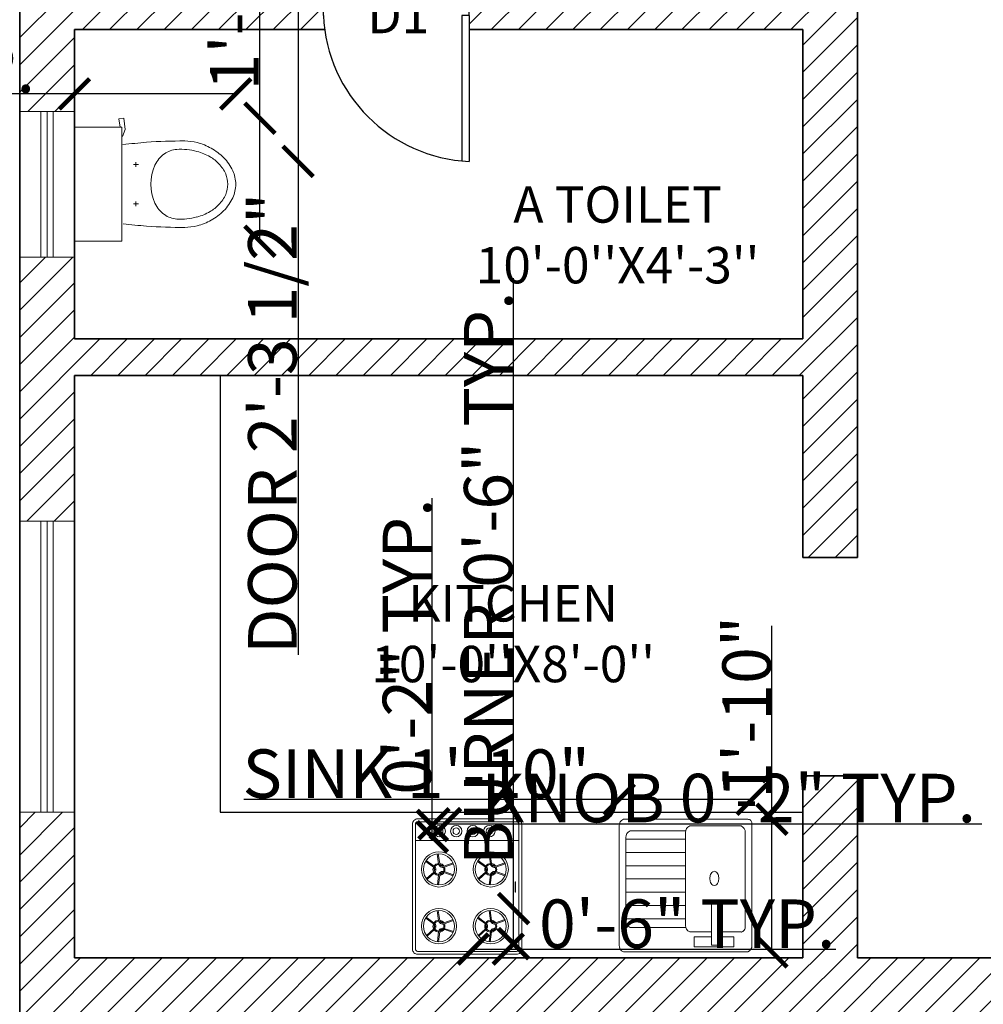
# Model space of a CAD drawing. Units: inches. Extents: x 2094 to 2639, y 1426 to 1997.
# Tile 3 of 8: x 2180 to 2339, y 1567 to 1730. Entities that reach past the tile are written whole.
import ezdxf

# ---------------------------------------------------------------- set-up
doc = ezdxf.new("R2010")
doc.units = ezdxf.units.IN
for name, color, linetype, lineweight in [('A-ANNO-DIMS', 2, 'Continuous', 18), ('A-ANNO-TEXT', 7, 'Continuous', 18), ('A-AREA-IDEN', 7, 'Continuous', 25), ('A-EQPM', 9, 'Continuous', 13), ('A-FLOR-FIXT', 9, 'Continuous', 18), ('A-WALL-PATT', 8, 'Continuous', 13), ('Doors', 34, 'Continuous', 25), ('Kitchen', 70, 'Continuous', 25), ('Walls', 7, 'Continuous', 35), ('Windows', 150, 'Continuous', 18)]:
    doc.layers.add(name, color=color, linetype=linetype, lineweight=lineweight)
doc.styles.get("Standard").update_dxf_attribs({"font": 'arial.ttf'})
doc.dimstyles.get("Standard").update_dxf_attribs({"dimtxt": 8, "dimasz": 5, "dimexe": 0.18, "dimexo": 0.0625, "dimgap": 0.09, "dimtad": 1, "dimdec": 1, "dimzin": 0, "dimdsep": 46, "dimlunit": 4, "dimtxsty": 'Standard', "dimblk": 'ARCHTICK', "dimcen": 0.09, "dimse1": 1, "dimse2": 1, "dimadec": 0, "dimazin": 0, "dimtfac": 1, "dimtdec": 1, "dimtofl": 0, "dimtmove": 0, "dimatfit": 3, "dimfxl": 1, "dimtolj": 1, "dimtzin": 0, "dimarcsym": 0})

# ---------------------------------------------------------------- blocks, each defined once
blk = doc.blocks.new('toilet-1')
at = {"color": 0, "linetype": 'ByBlock'}
for p, q in [((-0.23, -0.02), (-0.23, -0.2116)), ((0.23, -0.02), (-0.23, -0.02)), ((0.23, -0.02), (0.23, -0.2116)), ((-0.23, -0.2116), (0.23, -0.2116)), ((0.1917, -0.2144), (0.2206, -0.225)), ((0.2206, -0.225), (0.266, -0.2187)), ((0.2633, -0.1997), (0.23, -0.2044)), ((0.266, -0.2187), (0.2633, -0.1997)), ((-0.0889, -0.2683), (-0.0697, -0.2683)), ((-0.0793, -0.2587), (-0.0793, -0.2778)), ((0.0889, -0.2683), (0.0698, -0.2683)), ((0.0794, -0.2587), (0.0794, -0.2778)), ((0, -0.6382), (0, -0.6382))]:
    blk.add_line(p, q, dxfattribs=at)
for centre, radius, start, end in [((3.5272, -0.6239), 3.7093, 173.6925, 175.1593), ((-3.527, -0.624), 3.7093, 4.8413, 6.3171), ((1.7368, -0.4519), 1.9109, 175.7698, 180.3758), ((-1.7366, -0.4519), 1.9109, 359.6242, 4.2302), ((-0.0312, -0.4465), 0.1114, 113.8997, 145.1485), ((0, -0.5169), 0.1884, 66.0939, 113.9061), ((0.0312, -0.4465), 0.1114, 34.8515, 66.1003), ((-0.0408, -0.4398), 0.0996, 145.1497, 175.881), ((0.0409, -0.4398), 0.0996, 4.119, 34.8503), ((0.0981, -0.4497), 0.2389, 175.8862, 195.5931), ((-0.098, -0.4497), 0.2389, 344.4069, 4.1138), ((0.0353, -0.463), 0.2093, 180.3747, 194.3375), ((-0.0351, -0.463), 0.2093, 345.6614, 359.6243), ((0.055, -0.458), 0.2297, 194.3353, 209.622), ((0.0961, -0.4503), 0.2369, 195.5969, 209.3771), ((-0.096, -0.4503), 0.2369, 330.6229, 344.4031), ((-0.0548, -0.458), 0.2297, 330.3788, 345.6655), ((0.0647, -0.4524), 0.2409, 209.6273, 224.5489), ((0.0232, -0.4913), 0.1532, 209.3871, 226.5438), ((-0.0231, -0.4913), 0.1532, 313.4562, 330.6129), ((-0.0645, -0.4524), 0.2409, 315.4504, 330.372), ((0.0178, -0.4986), 0.1751, 224.552, 245.714), ((0.0152, -0.4997), 0.1416, 226.5501, 246.5527), ((0, -0.5347), 0.1034, 246.5493, 270.0042), ((0, -0.5347), 0.1034, 269.9958, 293.4507), ((-0.0151, -0.4997), 0.1416, 293.4473, 313.4499), ((-0.0176, -0.4986), 0.1751, 294.2865, 315.4485), ((0.0004, -0.538), 0.132, 245.5845, 269.8782), ((-0.0002, -0.538), 0.132, 270.1216, 294.4153)]:
    blk.add_arc(centre, radius, start, end, dxfattribs=at)
blk = doc.blocks.new('S_SINK12')
for p, q in [((0.25, 0.45), (0.25, 0.0004)), ((0.35, 0.45), (0.35, 0.0004)), ((0.45, 0.45), (0.45, 0.0004)), ((0.55, 0.45), (0.55, 0.0004)), ((0.65, 0.45), (0.65, 0.0004)), ((0.75, 0.45), (0.75, 0.0004)), ((0.85, 0.45), (0.85, 0.0004))]:
    blk.add_line(p, q)
for points in [[(0, -0.4688), (0, 0.4688, -0.310961), (0.05, 0.4998), (0.95, 0.4998, -0.310466), (1, 0.4686), (1, -0.4688, -0.414214), (0.9687, -0.5), (0.05, -0.5002, -0.309971)], [(0.0516, -0.1954), (0.0516, -0.242), (0.3617, -0.242, 1), (0.3617, -0.1954)], [(0.4997, -0.2171), (0.5033, -0.2291, 0.107136), (0.5156, -0.241, 0.076468), (0.5341, -0.249), (0.5538, -0.2509), (0.5755, -0.2481, 0.076468), (0.5921, -0.241, 0.107136), (0.6044, -0.2291), (0.608, -0.2171), (0.6044, -0.2051, 0.107136), (0.5921, -0.1931, 0.076468), (0.5755, -0.186), (0.5538, -0.1832), (0.5322, -0.186, 0.076468), (0.5156, -0.1931, 0.107136), (0.5033, -0.2051)]]:
    blk.add_lwpolyline(points, format="xyb", close=True)
for points in [[(0.1851, -0.001), (0.1851, 0.4188, -0.310466), (0.2351, 0.45), (0.8621, 0.45, -0.310466), (0.9121, 0.4188), (0.9121, -0.0005, -0.310466)], [(0.15, -0.1954), (0.15, -0.0308, -0.310466), (0.2, 0.0004), (0.9, 0.0004, -0.310466), (0.95, -0.0308), (0.95, -0.4189, -0.310466), (0.9, -0.4502), (0.2, -0.4502), (0.1799, -0.4479, -0.071009), (0.1646, -0.4419, -0.106323), (0.1531, -0.4318), (0.1499, -0.422), (0.1508, -0.4192)]]:
    blk.add_lwpolyline(points, format="xyb")
for points in [[(0.1136, -0.242), (0.1136, -0.3644), (0.0386, -0.3644), (0.0386, -0.0644), (0.1136, -0.0644), (0.1136, -0.1954)], [(0.15, -0.4189), (0.15, -0.242)]]:
    blk.add_lwpolyline(points)
blk = doc.blocks.new('AP0B05')
for p, q in [((35, 100), (35, 880)), ((75, 100), (75, 878.9)), ((35, 100), (35, -20)), ((815, 100), (815, -20))]:
    blk.add_line(p, q)
blk.add_lwpolyline([(35, 100), (75, 100)])
blk.add_arc((-2.4, 62.6), 818.3, 2.6212, 87.3788)
blk = doc.blocks.new('_ArchTick')
at = {"color": 0, "linetype": 'ByBlock', "const_width": 0.15}
blk.add_lwpolyline([(-0.5, -0.5), (0.5, 0.5)], dxfattribs=at)
blk = doc.blocks.new('*D14')
at = {"layer": 'A-ANNO-DIMS', "color": 0, "lineweight": -2, "transparency": 16777216}
blk.add_line((2154, 1928.9), (2154, 1459.9), dxfattribs=at)
at = {"layer": 'Defpoints', "color": 0, "transparency": 16777216}
for p in [(2180.06, 1928.9), (2154, 1459.9), (2180.06, 1459.9)]:
    blk.add_point(p, dxfattribs=at)
at = {"layer": 'A-ANNO-DIMS', "color": 0, "lineweight": -2, "transparency": 16777216, "xscale": 5, "yscale": 5, "zscale": 5}
for p, rotation in [((2154, 1928.9), 90), ((2154, 1459.9), 270)]:
    blk.add_blockref('_ArchTick', p, dxfattribs=dict(at, rotation=rotation))
at = {"layer": 'A-ANNO-DIMS', "color": 0, "transparency": 16777216, "insert": (2149.82, 1694.4), "char_height": 8, "attachment_point": 5, "rotation": 90}
blk.add_mtext('\\A1;39\'-1"', dxfattribs=at)
blk = doc.blocks.new('COOKTOP-BURNER')
for points in [[(-0.28, 2.54), (-0.05, 0.93, 0.472479), (0.86, 0.37), (2.39, 0.92)], [(-0.11, 2.56), (0.12, 0.95, 0.472071), (0.81, 0.53), (2.32, 1.08)], [(-2.06, -1.52), (-0.85, -0.44, 0.472071), (-0.89, 0.37), (-2.19, 1.33)], [(-1.95, -1.65), (-0.74, -0.56, 0.472479), (-0.79, 0.51), (-2.09, 1.47)], [(-0.26, -2.54), (-0.05, -0.93, -0.472479), (0.87, -0.36), (2.39, -0.9)], [(-0.09, -2.56), (0.12, -0.95, -0.472071), (0.81, -0.52), (2.33, -1.06)]]:
    blk.add_lwpolyline(points, format="xyb")
for radius in [2.9, 2.56]:
    blk.add_circle((0, 0), radius)
for radius, start, end in [(0.989, 156.9326, 207.478), (0.989, 93.6067, 146.9387), (0.818, 161.7394, 202.6344), (0.818, 92.012, 148.4601), (0.989, 33.0309, 83.5763), (0.818, 37.8377, 78.7328), (0.818, 335.9407, 24.5584), (0.989, 337.462, 23.0371), (0.989, 217.5084, 266.8924), (0.818, 215.9137, 268.4871), (0.989, 276.9228, 327.4682), (0.818, 281.7663, 322.6614)]:
    blk.add_arc((0, 0), radius, start, end)
blk = doc.blocks.new('COOKTOP-KNOB')
for radius in [0.938, 0.533]:
    blk.add_circle((0, 0), radius)
blk = doc.blocks.new('*D23')
at = {"layer": 'A-ANNO-DIMS', "color": 0, "lineweight": -2, "transparency": 16777216}
for p, q in [((2225.93, 1733.9), (2225.93, 1706.16)), ((2225.93, 1706.16), (2225.93, 1624.84))]:
    blk.add_line(p, q, dxfattribs=at)
at = {"layer": 'Defpoints', "color": 0, "transparency": 16777216}
for p in [(2230.09, 1733.9), (2225.93, 1706.16), (2230.09, 1706.16)]:
    blk.add_point(p, dxfattribs=at)
at = {"layer": 'A-ANNO-DIMS', "color": 0, "lineweight": -2, "transparency": 16777216, "xscale": 5, "yscale": 5, "zscale": 5}
for p, rotation in [((2225.93, 1733.9), 90), ((2225.93, 1706.16), 270)]:
    blk.add_blockref('_ArchTick', p, dxfattribs=dict(at, rotation=rotation))
at = {"layer": 'A-ANNO-DIMS', "color": 0, "transparency": 16777216, "insert": (2221.69, 1663), "char_height": 8, "attachment_point": 5, "rotation": 90}
blk.add_mtext('\\A1;DOOR 2\'-3 1/2"', dxfattribs=at)
blk = doc.blocks.new('*D39')
at = {"layer": 'A-ANNO-DIMS', "color": 0, "lineweight": -2, "transparency": 16777216}
for p, q in [((2189.06, 1717.27), (2094.42, 1717.27)), ((2215.64, 1717.27), (2189.06, 1717.27))]:
    blk.add_line(p, q, dxfattribs=at)
at = {"layer": 'Defpoints', "color": 0, "transparency": 16777216}
for p in [(2189.06, 1717.27), (2189.06, 1713.28), (2215.64, 1713.28)]:
    blk.add_point(p, dxfattribs=at)
at = {"layer": 'A-ANNO-DIMS', "color": 0, "lineweight": -2, "transparency": 16777216, "xscale": 5, "yscale": 5, "zscale": 5, "rotation": 180}
blk.add_blockref('_ArchTick', (2189.06, 1717.27), dxfattribs=at)
at = {"layer": 'A-ANNO-DIMS', "color": 0, "lineweight": -2, "transparency": 16777216, "xscale": 5, "yscale": 5, "zscale": 5}
blk.add_blockref('_ArchTick', (2215.64, 1717.27), dxfattribs=at)
at = {"layer": 'A-ANNO-DIMS', "color": 0, "transparency": 16777216, "insert": (2139.24, 1721.49), "char_height": 8, "attachment_point": 5}
blk.add_mtext('\\A1;WC 2\'-2 1/2" TYP.', dxfattribs=at)
blk = doc.blocks.new('*D40')
at = {"layer": 'A-ANNO-DIMS', "color": 0, "lineweight": -2, "transparency": 16777216}
for p, q in [((2219.63, 1713.28), (2219.63, 1785.11)), ((2219.63, 1692.99), (2219.63, 1713.28))]:
    blk.add_line(p, q, dxfattribs=at)
at = {"layer": 'Defpoints', "color": 0, "transparency": 16777216}
for p in [(2215.64, 1713.28), (2219.63, 1713.28), (2215.64, 1692.99)]:
    blk.add_point(p, dxfattribs=at)
at = {"layer": 'A-ANNO-DIMS', "color": 0, "lineweight": -2, "transparency": 16777216, "xscale": 5, "yscale": 5, "zscale": 5}
for p, rotation in [((2219.63, 1713.28), 90), ((2219.63, 1692.99), 270)]:
    blk.add_blockref('_ArchTick', p, dxfattribs=dict(at, rotation=rotation))
at = {"layer": 'A-ANNO-DIMS', "color": 0, "transparency": 16777216, "insert": (2215.41, 1751.7), "char_height": 8, "attachment_point": 5, "rotation": 90}
blk.add_mtext('\\A1;1\'-8 1/2" TYP.', dxfattribs=at)
blk = doc.blocks.new('*D41')
at = {"layer": 'A-ANNO-DIMS', "color": 0, "lineweight": -2, "transparency": 16777216}
for p, q in [((2261.42, 1583.02), (2261.42, 1686.91)), ((2261.42, 1577.23), (2261.42, 1583.02))]:
    blk.add_line(p, q, dxfattribs=at)
at = {"layer": 'Defpoints', "color": 0, "transparency": 16777216}
for p in [(2260.56, 1583.02), (2261.42, 1583.02), (2260.56, 1577.23)]:
    blk.add_point(p, dxfattribs=at)
at = {"layer": 'A-ANNO-DIMS', "color": 0, "lineweight": -2, "transparency": 16777216, "xscale": 5, "yscale": 5, "zscale": 5}
for p, rotation in [((2261.42, 1583.02), 90), ((2261.42, 1577.23), 270)]:
    blk.add_blockref('_ArchTick', p, dxfattribs=dict(at, rotation=rotation))
at = {"layer": 'A-ANNO-DIMS', "color": 0, "transparency": 16777216, "insert": (2257.25, 1637.47), "char_height": 8, "attachment_point": 5, "rotation": 90}
blk.add_mtext('\\A1;BURNER 0\'-6" TYP.', dxfattribs=at)
blk = doc.blocks.new('*D42')
at = {"layer": 'A-ANNO-DIMS', "color": 0, "lineweight": -2, "transparency": 16777216}
for p, q in [((2254.76, 1576.36), (2260.56, 1576.36)), ((2260.56, 1576.36), (2314.5, 1576.36))]:
    blk.add_line(p, q, dxfattribs=at)
at = {"layer": 'Defpoints', "color": 0, "transparency": 16777216}
for p in [(2254.76, 1577.23), (2260.56, 1577.23), (2260.56, 1576.36)]:
    blk.add_point(p, dxfattribs=at)
at = {"layer": 'A-ANNO-DIMS', "color": 0, "lineweight": -2, "transparency": 16777216, "xscale": 5, "yscale": 5, "zscale": 5, "rotation": 180}
blk.add_blockref('_ArchTick', (2254.76, 1576.36), dxfattribs=at)
at = {"layer": 'A-ANNO-DIMS', "color": 0, "lineweight": -2, "transparency": 16777216, "xscale": 5, "yscale": 5, "zscale": 5}
blk.add_blockref('_ArchTick', (2260.56, 1576.36), dxfattribs=at)
at = {"layer": 'A-ANNO-DIMS', "color": 0, "transparency": 16777216, "insert": (2290.03, 1580.53), "char_height": 8, "attachment_point": 5}
blk.add_mtext('\\A1;0\'-6" TYP.', dxfattribs=at)
blk = doc.blocks.new('*D43')
at = {"layer": 'A-ANNO-DIMS', "color": 0, "lineweight": -2, "transparency": 16777216}
for p, q in [((2248.31, 1597.01), (2250.19, 1597.01)), ((2250.19, 1597.01), (2338.56, 1597.01))]:
    blk.add_line(p, q, dxfattribs=at)
at = {"layer": 'Defpoints', "color": 0, "transparency": 16777216}
for p in [(2248.31, 1596.73), (2250.19, 1597.01), (2250.19, 1596.73)]:
    blk.add_point(p, dxfattribs=at)
at = {"layer": 'A-ANNO-DIMS', "color": 0, "lineweight": -2, "transparency": 16777216, "xscale": 5, "yscale": 5, "zscale": 5, "rotation": 180}
blk.add_blockref('_ArchTick', (2248.31, 1597.01), dxfattribs=at)
at = {"layer": 'A-ANNO-DIMS', "color": 0, "lineweight": -2, "transparency": 16777216, "xscale": 5, "yscale": 5, "zscale": 5}
blk.add_blockref('_ArchTick', (2250.19, 1597.01), dxfattribs=at)
at = {"layer": 'A-ANNO-DIMS', "color": 0, "transparency": 16777216, "insert": (2296.87, 1601.24), "char_height": 8, "attachment_point": 5}
blk.add_mtext('\\A1;KNOB 0\'-2" TYP.', dxfattribs=at)
blk = doc.blocks.new('*D44')
at = {"layer": 'A-ANNO-DIMS', "color": 0, "lineweight": -2, "transparency": 16777216}
for p, q in [((2248.03, 1596.73), (2248.03, 1650.68)), ((2248.03, 1594.86), (2248.03, 1596.73))]:
    blk.add_line(p, q, dxfattribs=at)
at = {"layer": 'Defpoints', "color": 0, "transparency": 16777216}
for p in [(2248.03, 1596.73), (2248.31, 1596.73), (2248.31, 1594.86)]:
    blk.add_point(p, dxfattribs=at)
at = {"layer": 'A-ANNO-DIMS', "color": 0, "lineweight": -2, "transparency": 16777216, "xscale": 5, "yscale": 5, "zscale": 5}
for p, rotation in [((2248.03, 1596.73), 90), ((2248.03, 1594.86), 270)]:
    blk.add_blockref('_ArchTick', p, dxfattribs=dict(at, rotation=rotation))
at = {"layer": 'A-ANNO-DIMS', "color": 0, "transparency": 16777216, "insert": (2243.86, 1626.2), "char_height": 8, "attachment_point": 5, "rotation": 90}
blk.add_mtext('\\A1;0\'-2" TYP.', dxfattribs=at)
blk = doc.blocks.new('*D45')
at = {"layer": 'A-ANNO-DIMS', "color": 0, "lineweight": -2, "transparency": 16777216}
for p, q in [((2278.81, 1601.03), (2217, 1601.03)), ((2300.71, 1601.03), (2278.81, 1601.03))]:
    blk.add_line(p, q, dxfattribs=at)
at = {"layer": 'Defpoints', "color": 0, "transparency": 16777216}
for p in [(2278.81, 1601.03), (2278.81, 1597.75), (2300.71, 1597.75)]:
    blk.add_point(p, dxfattribs=at)
at = {"layer": 'A-ANNO-DIMS', "color": 0, "lineweight": -2, "transparency": 16777216, "xscale": 5, "yscale": 5, "zscale": 5, "rotation": 180}
blk.add_blockref('_ArchTick', (2278.81, 1601.03), dxfattribs=at)
at = {"layer": 'A-ANNO-DIMS', "color": 0, "lineweight": -2, "transparency": 16777216, "xscale": 5, "yscale": 5, "zscale": 5}
blk.add_blockref('_ArchTick', (2300.71, 1601.03), dxfattribs=at)
at = {"layer": 'A-ANNO-DIMS', "color": 0, "transparency": 16777216, "insert": (2245.4, 1605.26), "char_height": 8, "attachment_point": 5}
blk.add_mtext('\\A1;SINK 1\'-10"', dxfattribs=at)
blk = doc.blocks.new('*D46')
at = {"layer": 'A-ANNO-DIMS', "color": 0, "lineweight": -2, "transparency": 16777216}
for p, q in [((2303.99, 1597.75), (2303.99, 1629.65)), ((2303.99, 1575.89), (2303.99, 1597.75))]:
    blk.add_line(p, q, dxfattribs=at)
at = {"layer": 'Defpoints', "color": 0, "transparency": 16777216}
for p in [(2300.71, 1597.75), (2303.99, 1597.75), (2300.71, 1575.89)]:
    blk.add_point(p, dxfattribs=at)
at = {"layer": 'A-ANNO-DIMS', "color": 0, "lineweight": -2, "transparency": 16777216, "xscale": 5, "yscale": 5, "zscale": 5}
for p, rotation in [((2303.99, 1597.75), 90), ((2303.99, 1575.89), 270)]:
    blk.add_blockref('_ArchTick', p, dxfattribs=dict(at, rotation=rotation))
at = {"layer": 'A-ANNO-DIMS', "color": 0, "transparency": 16777216, "insert": (2299.82, 1616.2), "char_height": 8, "attachment_point": 5, "rotation": 90}
blk.add_mtext('\\A1;1\'-10"', dxfattribs=at)
blk = doc.blocks.new('*D56')
at = {"layer": 'A-ANNO-DIMS', "color": 0, "lineweight": -2, "transparency": 16777216}
blk.add_line((2154.31, 1565.9), (2154.31, 1598.9), dxfattribs=at)
at = {"layer": 'Defpoints', "color": 0, "transparency": 16777216}
for p in [(2154.31, 1598.9), (2180.06, 1598.9), (2189.06, 1565.9)]:
    blk.add_point(p, dxfattribs=at)
at = {"layer": 'A-ANNO-DIMS', "color": 0, "lineweight": -2, "transparency": 16777216, "xscale": 5, "yscale": 5, "zscale": 5}
for p, rotation in [((2154.31, 1598.9), 90), ((2154.31, 1565.9), 270)]:
    blk.add_blockref('_ArchTick', p, dxfattribs=dict(at, rotation=rotation))
at = {"layer": 'A-ANNO-DIMS', "color": 0, "transparency": 16777216, "insert": (2150.13, 1582.4), "char_height": 8, "attachment_point": 5, "rotation": 90}
blk.add_mtext('\\A1;2\'-9"', dxfattribs=at)
blk = doc.blocks.new('*D65')
at = {"layer": 'A-ANNO-DIMS', "color": 0, "lineweight": -2, "transparency": 16777216}
blk.add_line((2562.81, 1604.9), (2562.81, 1640.9), dxfattribs=at)
at = {"layer": 'Defpoints', "color": 0, "transparency": 16777216}
for p in [(2318.06, 1640.9), (2562.81, 1640.9), (2318.06, 1604.9)]:
    blk.add_point(p, dxfattribs=at)
at = {"layer": 'A-ANNO-DIMS', "color": 0, "lineweight": -2, "transparency": 16777216, "xscale": 5, "yscale": 5, "zscale": 5}
for p, rotation in [((2562.81, 1640.9), 90), ((2562.81, 1604.9), 270)]:
    blk.add_blockref('_ArchTick', p, dxfattribs=dict(at, rotation=rotation))
at = {"layer": 'A-ANNO-DIMS', "color": 0, "transparency": 16777216, "insert": (2558.63, 1622.9), "char_height": 8, "attachment_point": 5, "rotation": 90}
blk.add_mtext('\\A1;3\'-0"', dxfattribs=at)
blk = doc.blocks.new('*D67')
at = {"layer": 'A-ANNO-DIMS', "color": 0, "lineweight": -2, "transparency": 16777216}
for p, q in [((2562.81, 1676.9), (2562.81, 1703.34)), ((2562.81, 1670.9), (2562.81, 1676.9))]:
    blk.add_line(p, q, dxfattribs=at)
at = {"layer": 'Defpoints', "color": 0, "transparency": 16777216}
for p in [(2309.06, 1676.9), (2562.81, 1676.9), (2309.06, 1670.9)]:
    blk.add_point(p, dxfattribs=at)
at = {"layer": 'A-ANNO-DIMS', "color": 0, "lineweight": -2, "transparency": 16777216, "xscale": 5, "yscale": 5, "zscale": 5}
for p, rotation in [((2562.81, 1676.9), 90), ((2562.81, 1670.9), 270)]:
    blk.add_blockref('_ArchTick', p, dxfattribs=dict(at, rotation=rotation))
at = {"layer": 'A-ANNO-DIMS', "color": 0, "transparency": 16777216, "insert": (2558.63, 1692.62), "char_height": 8, "attachment_point": 5, "rotation": 90}
blk.add_mtext('\\A1;0\'-6"', dxfattribs=at)
blk = doc.blocks.new('*D68')
at = {"layer": 'A-ANNO-DIMS', "color": 0, "lineweight": -2, "transparency": 16777216}
blk.add_line((2189.06, 1954.65), (2213.06, 1954.65), dxfattribs=at)
at = {"layer": 'Defpoints', "color": 0, "transparency": 16777216}
for p in [(2213.06, 1954.65), (2189.06, 1670.9), (2213.06, 1670.9)]:
    blk.add_point(p, dxfattribs=at)
at = {"layer": 'A-ANNO-DIMS', "color": 0, "lineweight": -2, "transparency": 16777216, "xscale": 5, "yscale": 5, "zscale": 5, "rotation": 180}
blk.add_blockref('_ArchTick', (2189.06, 1954.65), dxfattribs=at)
at = {"layer": 'A-ANNO-DIMS', "color": 0, "lineweight": -2, "transparency": 16777216, "xscale": 5, "yscale": 5, "zscale": 5}
blk.add_blockref('_ArchTick', (2213.06, 1954.65), dxfattribs=at)
at = {"layer": 'A-ANNO-DIMS', "color": 0, "transparency": 16777216, "insert": (2201.06, 1958.82), "char_height": 8, "attachment_point": 5}
blk.add_mtext('\\A1;2\'-0"', dxfattribs=at)
blk = doc.blocks.new('*D69')
at = {"layer": 'A-ANNO-DIMS', "color": 0, "lineweight": -2, "transparency": 16777216}
blk.add_line((2562.81, 1574.9), (2562.81, 1604.9), dxfattribs=at)
at = {"layer": 'Defpoints', "color": 0, "transparency": 16777216}
for p in [(2318.06, 1604.9), (2562.81, 1604.9), (2318.06, 1574.9)]:
    blk.add_point(p, dxfattribs=at)
at = {"layer": 'A-ANNO-DIMS', "color": 0, "lineweight": -2, "transparency": 16777216, "xscale": 5, "yscale": 5, "zscale": 5}
for p, rotation in [((2562.81, 1604.9), 90), ((2562.81, 1574.9), 270)]:
    blk.add_blockref('_ArchTick', p, dxfattribs=dict(at, rotation=rotation))
at = {"layer": 'A-ANNO-DIMS', "color": 0, "transparency": 16777216, "insert": (2558.63, 1589.9), "char_height": 8, "attachment_point": 5, "rotation": 90}
blk.add_mtext('\\A1;2\'-6"', dxfattribs=at)
blk = doc.blocks.new('*D71')
at = {"layer": 'A-ANNO-DIMS', "color": 0, "lineweight": -2, "transparency": 16777216}
for p, q in [((2300.69, 1434.15), (2309.06, 1434.15)), ((2309.06, 1434.15), (2354.14, 1434.15))]:
    blk.add_line(p, q, dxfattribs=at)
at = {"layer": 'Defpoints', "color": 0, "transparency": 16777216}
for p in [(2300.69, 1576.98), (2309.06, 1574.9), (2309.06, 1434.15)]:
    blk.add_point(p, dxfattribs=at)
at = {"layer": 'A-ANNO-DIMS', "color": 0, "lineweight": -2, "transparency": 16777216, "xscale": 5, "yscale": 5, "zscale": 5, "rotation": 180}
blk.add_blockref('_ArchTick', (2300.69, 1434.15), dxfattribs=at)
at = {"layer": 'A-ANNO-DIMS', "color": 0, "lineweight": -2, "transparency": 16777216, "xscale": 5, "yscale": 5, "zscale": 5}
blk.add_blockref('_ArchTick', (2309.06, 1434.15), dxfattribs=at)
at = {"layer": 'A-ANNO-DIMS', "color": 0, "transparency": 16777216, "insert": (2334.1, 1438.37), "char_height": 8, "attachment_point": 5}
blk.add_mtext('\\A1;0\'-8 1/2"', dxfattribs=at)
blk = doc.blocks.new('*D72')
at = {"layer": 'A-ANNO-DIMS', "color": 0, "lineweight": -2, "transparency": 16777216}
for p, q in [((2244.77, 1434.15), (2262.77, 1434.15)), ((2262.77, 1434.15), (2288.46, 1434.15))]:
    blk.add_line(p, q, dxfattribs=at)
at = {"layer": 'Defpoints', "color": 0, "transparency": 16777216}
for p in [(2244.77, 1576.36), (2262.77, 1576.36), (2262.77, 1434.15)]:
    blk.add_point(p, dxfattribs=at)
at = {"layer": 'A-ANNO-DIMS', "color": 0, "lineweight": -2, "transparency": 16777216, "xscale": 5, "yscale": 5, "zscale": 5, "rotation": 180}
blk.add_blockref('_ArchTick', (2244.77, 1434.15), dxfattribs=at)
at = {"layer": 'A-ANNO-DIMS', "color": 0, "lineweight": -2, "transparency": 16777216, "xscale": 5, "yscale": 5, "zscale": 5}
blk.add_blockref('_ArchTick', (2262.77, 1434.15), dxfattribs=at)
at = {"layer": 'A-ANNO-DIMS', "color": 0, "transparency": 16777216, "insert": (2278.12, 1438.32), "char_height": 8, "attachment_point": 5}
blk.add_mtext('\\A1;1\'-6"', dxfattribs=at)
blk = doc.blocks.new('*D73')
at = {"layer": 'A-ANNO-DIMS', "color": 0, "lineweight": -2, "transparency": 16777216}
for p, q in [((2262.77, 1434.15), (2278.83, 1434.15)), ((2278.83, 1434.15), (2304.53, 1434.15))]:
    blk.add_line(p, q, dxfattribs=at)
at = {"layer": 'Defpoints', "color": 0, "transparency": 16777216}
for p in [(2262.77, 1576.36), (2278.83, 1576.98), (2278.83, 1434.15)]:
    blk.add_point(p, dxfattribs=at)
at = {"layer": 'A-ANNO-DIMS', "color": 0, "lineweight": -2, "transparency": 16777216, "xscale": 5, "yscale": 5, "zscale": 5, "rotation": 180}
blk.add_blockref('_ArchTick', (2262.77, 1434.15), dxfattribs=at)
at = {"layer": 'A-ANNO-DIMS', "color": 0, "lineweight": -2, "transparency": 16777216, "xscale": 5, "yscale": 5, "zscale": 5}
blk.add_blockref('_ArchTick', (2278.83, 1434.15), dxfattribs=at)
at = {"layer": 'A-ANNO-DIMS', "color": 0, "transparency": 16777216, "insert": (2294.18, 1438.25), "char_height": 8, "attachment_point": 5}
blk.add_mtext('\\A1;1\'-4"', dxfattribs=at)
blk = doc.blocks.new('*D74')
at = {"layer": 'A-ANNO-DIMS', "color": 0, "lineweight": -2, "transparency": 16777216}
for p, q in [((2562.81, 1597.81), (2562.81, 1648.35)), ((2562.81, 1575.5), (2562.81, 1597.81))]:
    blk.add_line(p, q, dxfattribs=at)
at = {"layer": 'Defpoints', "color": 0, "transparency": 16777216}
for p in [(2261.92, 1597.81), (2562.81, 1597.81), (2261.92, 1575.5)]:
    blk.add_point(p, dxfattribs=at)
at = {"layer": 'A-ANNO-DIMS', "color": 0, "lineweight": -2, "transparency": 16777216, "xscale": 5, "yscale": 5, "zscale": 5}
for p, rotation in [((2562.81, 1597.81), 90), ((2562.81, 1575.5), 270)]:
    blk.add_blockref('_ArchTick', p, dxfattribs=dict(at, rotation=rotation))
at = {"layer": 'A-ANNO-DIMS', "color": 0, "transparency": 16777216, "insert": (2558.58, 1625.58), "char_height": 8, "attachment_point": 5, "rotation": 90}
blk.add_mtext('\\A1;1\'-10 1/2"', dxfattribs=at)
blk = doc.blocks.new('*D76')
at = {"layer": 'A-ANNO-DIMS', "color": 0, "lineweight": -2, "transparency": 16777216}
blk.add_line((2248.06, 1954.65), (2318.06, 1954.65), dxfattribs=at)
at = {"layer": 'Defpoints', "color": 0, "transparency": 16777216}
for p in [(2318.06, 1954.65), (2248.06, 1468.9), (2318.06, 1468.9)]:
    blk.add_point(p, dxfattribs=at)
at = {"layer": 'A-ANNO-DIMS', "color": 0, "lineweight": -2, "transparency": 16777216, "xscale": 5, "yscale": 5, "zscale": 5, "rotation": 180}
blk.add_blockref('_ArchTick', (2248.06, 1954.65), dxfattribs=at)
at = {"layer": 'A-ANNO-DIMS', "color": 0, "lineweight": -2, "transparency": 16777216, "xscale": 5, "yscale": 5, "zscale": 5}
blk.add_blockref('_ArchTick', (2318.06, 1954.65), dxfattribs=at)
at = {"layer": 'A-ANNO-DIMS', "color": 0, "transparency": 16777216, "insert": (2283.06, 1958.82), "char_height": 8, "attachment_point": 5}
blk.add_mtext('\\A1;5\'-10"', dxfattribs=at)
blk = doc.blocks.new('*D77')
at = {"layer": 'A-ANNO-DIMS', "color": 0, "lineweight": -2, "transparency": 16777216}
for p, q in [((2308.06, 1954.65), (2318.06, 1954.65)), ((2318.06, 1954.65), (2350.72, 1954.65))]:
    blk.add_line(p, q, dxfattribs=at)
at = {"layer": 'Defpoints', "color": 0, "transparency": 16777216}
for p in [(2318.06, 1954.65), (2308.06, 1468.9), (2318.06, 1468.9)]:
    blk.add_point(p, dxfattribs=at)
at = {"layer": 'A-ANNO-DIMS', "color": 0, "lineweight": -2, "transparency": 16777216, "xscale": 5, "yscale": 5, "zscale": 5, "rotation": 180}
blk.add_blockref('_ArchTick', (2308.06, 1954.65), dxfattribs=at)
at = {"layer": 'A-ANNO-DIMS', "color": 0, "lineweight": -2, "transparency": 16777216, "xscale": 5, "yscale": 5, "zscale": 5}
blk.add_blockref('_ArchTick', (2318.06, 1954.65), dxfattribs=at)
at = {"layer": 'A-ANNO-DIMS', "color": 0, "transparency": 16777216, "insert": (2336.89, 1958.82), "char_height": 8, "attachment_point": 5}
blk.add_mtext('\\A1;0\'-10"', dxfattribs=at)
blk = doc.blocks.new('*D81')
at = {"layer": 'A-ANNO-DIMS', "color": 0, "lineweight": -2, "transparency": 16777216}
for p, q in [((2249.13, 1954.65), (2257.66, 1954.65)), ((2257.66, 1954.65), (2302.74, 1954.65))]:
    blk.add_line(p, q, dxfattribs=at)
at = {"layer": 'Defpoints', "color": 0, "transparency": 16777216}
for p in [(2257.66, 1954.65), (2249.13, 1589.48), (2257.66, 1589.48)]:
    blk.add_point(p, dxfattribs=at)
at = {"layer": 'A-ANNO-DIMS', "color": 0, "lineweight": -2, "transparency": 16777216, "xscale": 5, "yscale": 5, "zscale": 5, "rotation": 180}
blk.add_blockref('_ArchTick', (2249.13, 1954.65), dxfattribs=at)
at = {"layer": 'A-ANNO-DIMS', "color": 0, "lineweight": -2, "transparency": 16777216, "xscale": 5, "yscale": 5, "zscale": 5}
blk.add_blockref('_ArchTick', (2257.66, 1954.65), dxfattribs=at)
at = {"layer": 'A-ANNO-DIMS', "color": 0, "transparency": 16777216, "insert": (2282.7, 1958.87), "char_height": 8, "attachment_point": 5}
blk.add_mtext('\\A1;0\'-8 1/2"', dxfattribs=at)
blk = doc.blocks.new('*D82')
at = {"layer": 'A-ANNO-DIMS', "color": 0, "lineweight": -2, "transparency": 16777216}
for p, q in [((2154.31, 1589.48), (2154.31, 1634.57)), ((2154.31, 1580.13), (2154.31, 1589.48))]:
    blk.add_line(p, q, dxfattribs=at)
at = {"layer": 'Defpoints', "color": 0, "transparency": 16777216}
for p in [(2154.31, 1589.48), (2249.13, 1589.48), (2249.13, 1580.13)]:
    blk.add_point(p, dxfattribs=at)
at = {"layer": 'A-ANNO-DIMS', "color": 0, "lineweight": -2, "transparency": 16777216, "xscale": 5, "yscale": 5, "zscale": 5}
for p, rotation in [((2154.31, 1589.48), 90), ((2154.31, 1580.13), 270)]:
    blk.add_blockref('_ArchTick', p, dxfattribs=dict(at, rotation=rotation))
at = {"layer": 'A-ANNO-DIMS', "color": 0, "transparency": 16777216, "insert": (2150.08, 1614.53), "char_height": 8, "attachment_point": 5, "rotation": 90}
blk.add_mtext('\\A1;0\'-9 1/2"', dxfattribs=at)
blk = doc.blocks.new('*D83')
at = {"layer": 'A-ANNO-DIMS', "color": 0, "lineweight": -2, "transparency": 16777216}
for p, q in [((2249.25, 1954.65), (2257.43, 1954.65)), ((2257.43, 1954.65), (2283.88, 1954.65))]:
    blk.add_line(p, q, dxfattribs=at)
at = {"layer": 'Defpoints', "color": 0, "transparency": 16777216}
for p in [(2257.43, 1954.65), (2249.25, 1595.79), (2257.43, 1595.79)]:
    blk.add_point(p, dxfattribs=at)
at = {"layer": 'A-ANNO-DIMS', "color": 0, "lineweight": -2, "transparency": 16777216, "xscale": 5, "yscale": 5, "zscale": 5, "rotation": 180}
blk.add_blockref('_ArchTick', (2249.25, 1954.65), dxfattribs=at)
at = {"layer": 'A-ANNO-DIMS', "color": 0, "lineweight": -2, "transparency": 16777216, "xscale": 5, "yscale": 5, "zscale": 5}
blk.add_blockref('_ArchTick', (2257.43, 1954.65), dxfattribs=at)
at = {"layer": 'A-ANNO-DIMS', "color": 0, "transparency": 16777216, "insert": (2273.16, 1958.82), "char_height": 8, "attachment_point": 5}
blk.add_mtext('\\A1;0\'-8"', dxfattribs=at)

msp = doc.modelspace()

# ---------------------------------------------------------------- hatches: boundary and pattern name
at = {"layer": 'A-WALL-PATT', "transparency": 33554585}
h = msp.add_hatch(dxfattribs=at)
h.set_pattern_fill('ANSI31', color=256)
h.paths.add_polyline_path([(2189.06, 1727.9), (2230.3, 1727.9, -0.022928), (2230.09, 1730.2), (2230.09, 1733.9), (2189.06, 1733.9), (2189.06, 1742.37), (2180.06, 1742.37), (2180.06, 1714.4), (2189.06, 1714.4)])
h.paths.add_polyline_path([(2456.51, 1574.9), (2413.83, 1574.9), (2413.83, 1565.9), (2456.51, 1565.9)])
h.paths.add_polyline_path([(2537.06, 1643.81), (2528.06, 1643.81), (2528.06, 1574.9), (2519.78, 1574.9), (2519.78, 1571.88), (2519.78, 1565.9), (2537.06, 1565.9)])
h.paths.add_polyline_path([(2339.06, 1928.9), (2300.94, 1928.9), (2300.94, 1919.9), (2309.06, 1919.9), (2309.06, 1776.3, -0.024186), (2312.62, 1776.64), (2318.06, 1776.64), (2318.06, 1778.9), (2336.06, 1778.9), (2336.06, 1787.9), (2318.06, 1787.9), (2318.06, 1835.9), (2384.06, 1835.9), (2384.06, 1787.9), (2366.06, 1787.9), (2366.06, 1778.9), (2479.64, 1778.9), (2479.64, 1784.88, -0.018603), (2479.89, 1787.9), (2390.06, 1787.9), (2390.06, 1847.57), (2385.61, 1847.57), (2384.06, 1847.57), (2384.06, 1841.9), (2318.06, 1841.9), (2318.06, 1919.9), (2339.06, 1919.9)])
h.paths.add_polyline_path([(2252.94, 1928.9), (2180.06, 1928.9), (2180.06, 1790.37), (2189.06, 1790.37), (2189.06, 1843.77), (2189.06, 1919.9), (2252.94, 1919.9)])
h.paths.add_polyline_path([(2472.33, 1928.9), (2363.06, 1928.9), (2363.06, 1919.9), (2384.06, 1919.9), (2384.06, 1876.38, -0.012802), (2385.61, 1876.49), (2390.06, 1876.49), (2390.06, 1919.9), (2472.33, 1919.9)], flags=17)
h.paths.add_polyline_path([(2537.06, 1928.9), (2520.33, 1928.9), (2520.33, 1919.9), (2528.06, 1919.9), (2528.06, 1905.95), (2528.06, 1787.9), (2518.5, 1787.9), (2518.5, 1784.88), (2518.5, 1778.9), (2528.06, 1778.9), (2528.06, 1715.81), (2537.06, 1715.81)])
h.paths.add_polyline_path([(2379.33, 1857.12), (2393.06, 1857.12), (2393.06, 1866.16), (2379.33, 1866.16)], flags=25)
h.paths.add_polyline_path([(2235.85, 1725.77), (2249.57, 1725.77), (2249.57, 1734.81), (2235.85, 1734.81)], flags=25)
h.paths.add_polyline_path([(2305.79, 1754.6), (2314.84, 1754.6), (2314.84, 1763.6), (2305.79, 1763.6)], flags=9)
h.paths.add_polyline_path([(2493.85, 1778.22), (2502.9, 1778.22), (2502.9, 1787.22), (2493.85, 1787.22)], flags=9)
h.paths.add_polyline_path([(2370.69, 1555.65), (2381.6, 1555.65), (2381.6, 1564.65), (2370.69, 1564.65)], flags=9)
h.paths.add_polyline_path([(2461.57, 1555.65), (2477.6, 1555.65), (2477.6, 1564.65), (2461.57, 1564.65)], flags=9)
h.paths.add_polyline_path([(2493.18, 1565.15), (2509.22, 1565.15), (2509.22, 1574.15), (2493.18, 1574.15)], flags=9)
h.paths.add_polyline_path([(2408.32, 1501.7), (2449.12, 1501.7), (2449.12, 1520.36), (2408.32, 1520.36)], flags=9)
h.paths.add_polyline_path([(2398.49, 1698.6), (2441.61, 1698.6), (2441.61, 1717.26), (2398.49, 1717.26)], flags=9)
h.paths.add_polyline_path([(2248.63, 1683.29), (2287.87, 1683.29), (2287.87, 1701.95), (2248.63, 1701.95)], flags=25)
h.paths.add_polyline_path([(2440.73, 1823.2), (2483.86, 1823.2), (2483.86, 1841.85), (2440.73, 1841.85)], flags=9)
h.paths.add_polyline_path([(2335.3, 1804.5), (2370.65, 1804.5), (2370.65, 1823.15), (2335.3, 1823.15)], flags=25)
h.paths.add_polyline_path([(2335.3, 1893.12), (2370.65, 1893.12), (2370.65, 1911.77), (2335.3, 1911.77)], flags=25)
h.paths.add_polyline_path([(2241.82, 1863.6), (2290.11, 1863.6), (2290.11, 1882.25), (2241.82, 1882.25)], flags=9)
h = msp.add_hatch(dxfattribs=at)
h.set_pattern_fill('ANSI31', color=256)
h.paths.add_polyline_path([(2318.06, 1741.32), (2312.62, 1741.32), (2309.06, 1741.32), (2309.06, 1733.9), (2254.12, 1733.9), (2254.12, 1730.2), (2254.12, 1727.9), (2309.06, 1727.9), (2309.06, 1676.9), (2189.06, 1676.9), (2189.06, 1690.4), (2180.06, 1690.4), (2180.06, 1646.9), (2189.06, 1646.9), (2189.06, 1670.9), (2309.06, 1670.9), (2309.06, 1640.9), (2318.06, 1640.9)])
h.paths.add_polyline_path([(2318.06, 1604.9), (2309.06, 1604.9), (2309.06, 1574.9), (2189.06, 1574.9), (2189.06, 1598.9), (2180.06, 1598.9), (2180.06, 1459.9), (2318.06, 1459.9), (2318.06, 1468.9), (2189.06, 1468.9), (2189.06, 1565.9), (2341.83, 1565.9), (2341.83, 1574.9), (2318.06, 1574.9)])

# ---------------------------------------------------------------- linework, layer by layer
at = {"layer": 'A-EQPM'}
msp.add_line((2262.29, 1594.26), (2245.24, 1594.26), dxfattribs=at)
for points in [[(2244.77, 1576.36), (2244.77, 1596.95, -0.414214), (2245.62, 1597.81), (2261.92, 1597.81, -0.414214), (2262.77, 1596.95), (2262.77, 1576.36, -0.414214), (2261.92, 1575.5), (2245.62, 1575.5, -0.414214)], [(2245.24, 1576.36), (2245.24, 1596.95, -0.414214), (2245.62, 1597.33), (2261.92, 1597.33, -0.414214), (2262.29, 1596.95), (2262.29, 1576.36, -0.414214), (2261.92, 1575.98), (2245.62, 1575.98, -0.414214)]]:
    msp.add_lwpolyline(points, format="xyb", close=True, dxfattribs=at)
msp.add_lwpolyline([(2261.75, 1587.44), (2261.75, 1585.73), (2261.68, 1585.73), (2261.68, 1587.44)], close=True, dxfattribs=at)
at = {"layer": 'Kitchen'}
for p, q in [((2213.06, 1670.9), (2213.06, 1598.9)), ((2213.06, 1598.9), (2309.06, 1598.9))]:
    msp.add_line(p, q, dxfattribs=at)
at = {"layer": 'Walls'}
for p, q in [((2180.06, 1928.9), (2180.06, 1459.9)), ((2318.06, 1741.32), (2318.06, 1640.9)), ((2189.06, 1727.9), (2230.3, 1727.9)), ((2189.06, 1727.9), (2189.06, 1676.9)), ((2254.12, 1727.9), (2309.06, 1727.9)), ((2309.06, 1727.9), (2309.06, 1676.9)), ((2189.06, 1676.9), (2309.06, 1676.9)), ((2189.06, 1670.9), (2309.06, 1670.9)), ((2189.06, 1670.9), (2189.06, 1574.9)), ((2309.06, 1670.9), (2309.06, 1640.9)), ((2309.06, 1640.9), (2318.06, 1640.9)), ((2309.06, 1604.9), (2318.06, 1604.9)), ((2309.06, 1604.9), (2309.06, 1574.9)), ((2318.06, 1604.9), (2318.06, 1574.9)), ((2189.06, 1574.9), (2309.06, 1574.9)), ((2318.06, 1574.9), (2481.17, 1574.9))]:
    msp.add_line(p, q, dxfattribs=at)
at = {"layer": 'Windows'}
for p, q in [((2183.56, 1690.4), (2183.56, 1714.4)), ((2184.56, 1690.4), (2184.56, 1714.4)), ((2185.56, 1690.4), (2185.56, 1714.4)), ((2183.56, 1598.9), (2183.56, 1646.9)), ((2184.56, 1598.9), (2184.56, 1646.9)), ((2185.56, 1598.9), (2185.56, 1646.9))]:
    msp.add_line(p, q, dxfattribs=at)
for points in [[(2189.06, 1690.4), (2189.06, 1714.4), (2180.06, 1714.4), (2180.06, 1690.4)], [(2189.06, 1598.9), (2189.06, 1646.9), (2180.06, 1646.9), (2180.06, 1598.9)]]:
    msp.add_lwpolyline(points, close=True, dxfattribs=at)

# ---------------------------------------------------------------- block references
at = {"layer": 'A-EQPM'}
for name, p in [('COOKTOP-KNOB', (2249.25, 1595.79)), ('COOKTOP-KNOB', (2251.98, 1595.79)), ('COOKTOP-KNOB', (2254.71, 1595.79)), ('COOKTOP-KNOB', (2257.43, 1595.79)), ('COOKTOP-BURNER', (2249.13, 1589.48)), ('COOKTOP-BURNER', (2257.66, 1589.48)), ('COOKTOP-BURNER', (2249.13, 1580.13)), ('COOKTOP-BURNER', (2257.66, 1580.13))]:
    msp.add_blockref(name, p, dxfattribs=at)
at = {"layer": 'A-FLOR-FIXT', "rotation": 90}
for name, p, xscale, yscale, zscale in [('toilet-1', (2188.24, 1702.4), 40.90426662806183, 40.90426662806183, 40.90426662806183), ('S_SINK12', (2289.76, 1575.89), 21.85587950619759, 21.85587950619759, 21.85587950619759)]:
    msp.add_blockref(name, p, dxfattribs=dict(at, xscale=xscale, yscale=yscale, zscale=zscale))
at = {"layer": 'Doors', "xscale": 0.0308176600246466, "yscale": 0.0308176600246466, "zscale": 0.0308176600246466, "rotation": 180}
msp.add_blockref('AP0B05', (2255.2, 1733.28), dxfattribs=at)

# ---------------------------------------------------------------- texts
at = {"layer": 'A-ANNO-TEXT'}
msp.add_text('D1', height=6, dxfattribs=at).set_placement((2237.35, 1727.28))
at = {"layer": 'A-AREA-IDEN', "char_height": 6, "attachment_point": 1}
for s, insert in [("\\pxqc;A TOILET\\P10'-0''X4'-3''", (2252.01, 1702.06)), ("\\pxqc;KITCHEN\\P10'-0''X8'-0''", (2234.8, 1636.33))]:
    msp.add_mtext_dynamic_manual_height_columns(s, width=53.0999, gutter_width=63.55, heights=[0], dxfattribs=dict(at, insert=insert))

# ---------------------------------------------------------------- dimensions: what is measured, and where the dimension line sits
at = {"layer": 'A-ANNO-DIMS'}
for base, p1, p2, picture, middle in [((2257.66, 1954.65), (2249.13, 1589.48), (2257.66, 1589.48), '*D81', (2282.7, 1958.87)), ((2213.06, 1954.65), (2189.06, 1670.9), (2213.06, 1670.9), '*D68', (2201.06, 1958.82)), ((2318.06, 1954.65), (2248.06, 1468.9), (2318.06, 1468.9), '*D76', (2283.06, 1958.82)), ((2257.43, 1954.65), (2249.25, 1595.79), (2257.43, 1595.79), '*D83', (2273.16, 1958.82)), ((2318.06, 1954.65), (2308.06, 1468.9), (2318.06, 1468.9), '*D77', (2336.89, 1958.82)), ((2262.77, 1434.15), (2244.77, 1576.36), (2262.77, 1576.36), '*D72', (2278.12, 1438.32)), ((2278.83, 1434.15), (2262.77, 1576.36), (2278.83, 1576.98), '*D73', (2294.18, 1438.25)), ((2309.06, 1434.15), (2300.69, 1576.98), (2309.06, 1574.9), '*D71', (2334.1, 1438.37))]:
    dim = msp.add_linear_dim(base=base, p1=p1, p2=p2, dimstyle='Standard', override={"dimdec": 1, "dimlfac": 1, "dimrnd": 0, "dimzin": 1, "dimdsep": 46, "dimlunit": 4, "dimfrac": 2}, dxfattribs=at)
    dim.commit()
    dim.dimension.update_dxf_attribs({"geometry": picture, "text_midpoint": middle})
for base, p1, p2, override, picture, middle in [((2154, 1459.9), (2180.06, 1928.9), (2180.06, 1459.9), {"dimclrd": 0, "dimclre": 0, "dimclrt": 0}, '*D14', (2149.82, 1694.4)), ((2562.81, 1676.9), (2309.06, 1670.9), (2309.06, 1676.9), {"dimdec": 1, "dimlfac": 1, "dimrnd": 0, "dimzin": 1, "dimdsep": 46, "dimlunit": 4, "dimfrac": 2}, '*D67', (2558.63, 1692.62)), ((2562.81, 1597.81), (2261.92, 1575.5), (2261.92, 1597.81), {"dimdec": 1, "dimlfac": 1, "dimrnd": 0, "dimzin": 1, "dimdsep": 46, "dimlunit": 4, "dimfrac": 2}, '*D74', (2558.58, 1625.58)), ((2562.81, 1640.9), (2318.06, 1604.9), (2318.06, 1640.9), {"dimdec": 1, "dimlfac": 1, "dimrnd": 0, "dimzin": 1, "dimdsep": 46, "dimlunit": 4, "dimfrac": 2}, '*D65', (2558.63, 1622.9)), ((2154.3063, 1589.4845), (2249.1311, 1580.1261), (2249.1311, 1589.4845), {"dimdec": 1, "dimlfac": 1, "dimrnd": 0, "dimzin": 1, "dimdsep": 46, "dimlunit": 4, "dimfrac": 2}, '*D82', (2150.0799, 1614.5281)), ((2303.99, 1597.75), (2300.71, 1575.89), (2300.71, 1597.75), {"dimdec": 1, "dimlfac": 1, "dimrnd": 0, "dimzin": 1, "dimdsep": 46, "dimlunit": 4, "dimfrac": 2}, '*D46', (2299.82, 1616.2)), ((2562.81, 1604.9), (2318.06, 1574.9), (2318.06, 1604.9), {"dimdec": 1, "dimlfac": 1, "dimrnd": 0, "dimzin": 1, "dimdsep": 46, "dimlunit": 4, "dimfrac": 2}, '*D69', (2558.63, 1589.9)), ((2154.31, 1598.9), (2189.06, 1565.9), (2180.06, 1598.9), {"dimdec": 1, "dimlfac": 1, "dimrnd": 0, "dimzin": 1, "dimdsep": 46, "dimlunit": 4, "dimfrac": 2}, '*D56', (2150.13, 1582.4))]:
    dim = msp.add_linear_dim(base=base, p1=p1, p2=p2, angle=90, dimstyle='Standard', override=override, dxfattribs=at)
    dim.commit()
    dim.dimension.update_dxf_attribs({"geometry": picture, "text_midpoint": middle})
for base, p1, p2, angle, text, picture, middle in [((2219.63, 1713.28), (2215.64, 1692.99), (2215.64, 1713.28), 90, '<> TYP.', '*D40', (2215.41, 1751.7)), ((2189.06, 1717.27), (2215.64, 1713.28), (2189.06, 1713.28), 180, 'WC <> TYP.', '*D39', (2139.24, 1721.49)), ((2225.93, 1706.16), (2230.09, 1733.9), (2230.09, 1706.16), 270, 'DOOR <>', '*D23', (2221.69, 1663)), ((2261.42, 1583.02), (2260.56, 1577.23), (2260.56, 1583.02), 90, 'BURNER <> TYP.', '*D41', (2257.25, 1637.47)), ((2248.03, 1596.73), (2248.31, 1594.86), (2248.31, 1596.73), 90, '<> TYP.', '*D44', (2243.86, 1626.2)), ((2278.81, 1601.03), (2300.71, 1597.75), (2278.81, 1597.75), 180, 'SINK <>', '*D45', (2245.4, 1605.26))]:
    dim = msp.add_linear_dim(base=base, p1=p1, p2=p2, angle=angle, text=text, dimstyle='Standard', override={"dimdec": 1, "dimlfac": 1, "dimrnd": 0, "dimzin": 1, "dimdsep": 46, "dimlunit": 4, "dimfrac": 2}, dxfattribs=at)
    dim.commit()
    dim.dimension.update_dxf_attribs({"geometry": picture, "text_midpoint": middle})
for base, p1, p2, text, picture, middle in [((2250.19, 1597.01), (2248.31, 1596.73), (2250.19, 1596.73), 'KNOB <> TYP.', '*D43', (2296.87, 1601.24)), ((2260.56, 1576.36), (2254.76, 1577.23), (2260.56, 1577.23), '<> TYP.', '*D42', (2290.03, 1580.53))]:
    dim = msp.add_linear_dim(base=base, p1=p1, p2=p2, text=text, dimstyle='Standard', override={"dimdec": 1, "dimlfac": 1, "dimrnd": 0, "dimzin": 1, "dimdsep": 46, "dimlunit": 4, "dimfrac": 2}, dxfattribs=at)
    dim.commit()
    dim.dimension.update_dxf_attribs({"geometry": picture, "text_midpoint": middle})

doc.saveas('drawing.dxf')
